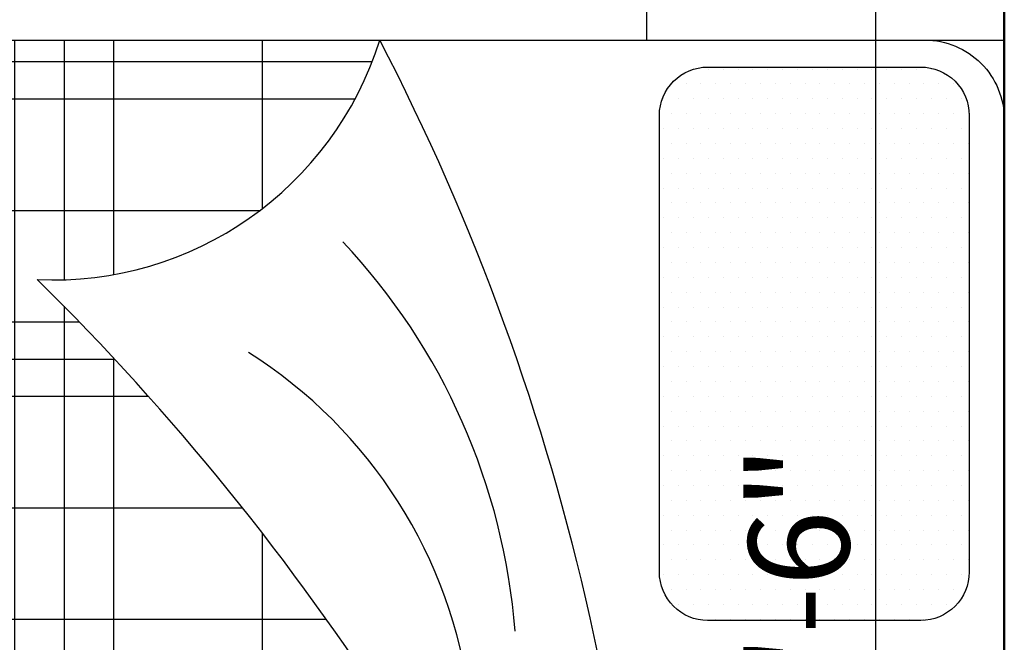
# Model space of a CAD drawing. Units: inches. Extents: x 3064 to 19385, y 846 to 15425.
# Tile 97 of 108: x 7612 to 7661, y 1063 to 1094. Entities that reach past the tile are written whole.
import ezdxf

# ---------------------------------------------------------------- set-up
doc = ezdxf.new("R2010")
doc.units = ezdxf.units.IN
for name, color, linetype, lineweight in [('A-ANNO-DIMS', 2, 'Continuous', 18), ('A-FLOR-FIXT', 9, 'Continuous', 18), ('A-WALL', 7, 'Continuous', 50)]:
    doc.layers.add(name, color=color, linetype=linetype, lineweight=lineweight)
doc.layers.add('BLOCK', color=6, linetype='Continuous')
doc.styles.get("Standard").update_dxf_attribs({"font": 'arial.ttf'})
doc.dimstyles.new('ISO-25', dxfattribs={"dimtxt": 9, "dimasz": 2.5, "dimexe": 1.25, "dimexo": 0.625, "dimtad": 1, "dimdec": 1, "dimlunit": 3, "dimtxsty": 'Standard', "dimcen": 2.5, "dimadec": 0, "dimazin": 0, "dimtfac": 1, "dimtdec": 1, "dimtmove": 0, "dimatfit": 3, "dimfxl": 1, "dimarcsym": 0})

# ---------------------------------------------------------------- blocks, each defined once
blk = doc.blocks.new('*D234')
at = {"layer": 'A-ANNO-DIMS', "color": 0, "lineweight": -2, "transparency": 16777216}
for p, q in [((7660.621, 1144.34), (7653.626, 1144.34)), ((7654.876, 984.84), (7654.876, 1141.84)), ((7660.621, 982.34), (7653.626, 982.34))]:
    blk.add_line(p, q, dxfattribs=at)
at = {"layer": 'A-ANNO-DIMS', "color": 0, "transparency": 16777216}
for points in [[(7654.459, 1141.84), (7655.292, 1141.84), (7654.876, 1144.34)], [(7654.459, 984.84), (7655.292, 984.84), (7654.876, 982.34)]]:
    blk.add_solid(points, dxfattribs=at)
at = {"layer": 'Defpoints', "color": 0, "transparency": 16777216}
for p in [(7654.876, 1144.34), (7661.246, 1144.34), (7661.246, 982.34)]:
    blk.add_point(p, dxfattribs=at)
at = {"layer": 'A-ANNO-DIMS', "color": 0, "transparency": 16777216, "insert": (7651.696, 1063.34), "char_height": 5, "attachment_point": 5, "rotation": 90}
blk.add_mtext('13\'-6"', dxfattribs=at)
blk = doc.blocks.new('*X5')
at = {"color": 0}
for p, q in [((276.598, 451.25), (280.51, 451.25)), ((275.455, 450.625), (280.51, 450.625)), ((274.411, 450), (280.51, 450)), ((265.51, 448.125), (267.634, 448.125)), ((271.723, 448.125), (280.51, 448.125)), ((265.51, 446.25), (268.465, 446.25)), ((269.519, 446.25), (280.51, 446.25)), ((265.51, 445.625), (268.531, 445.625)), ((268.866, 445.625), (280.51, 445.625)), ((265.51, 445), (280.51, 445)), ((265.51, 443.125), (280.51, 443.125)), ((265.51, 441.25), (280.51, 441.25)), ((265.51, 440.625), (280.51, 440.625)), ((265.634, 440), (280.386, 440))]:
    blk.add_line(p, q, dxfattribs=at)
blk = doc.blocks.new('*X6')
at = {"color": 0}
for p, q in [((265.781, 439.797), (265.781, 449.511)), ((266.25, 439.517), (266.25, 449.296)), ((272.812, 439.482), (272.812, 448.934)), ((267.656, 439.482), (267.656, 448.095)), ((271.406, 439.482), (271.406, 447.876)), ((270, 439.482), (270, 446.689)), ((269.531, 439.482), (269.531, 446.262)), ((269.062, 439.482), (269.062, 445.817))]:
    blk.add_line(p, q, dxfattribs=at)
blk = doc.blocks.new('*X7')
at = {"color": 0}
for p, q in [((266.4375, 457.03125), (266.4375, 457.03125)), ((266.8125, 457.03125), (266.8125, 457.03125)), ((267.1875, 457.03125), (267.1875, 457.03125)), ((267.5625, 457.03125), (267.5625, 457.03125)), ((267.9375, 457.03125), (267.9375, 457.03125)), ((268.3125, 457.03125), (268.3125, 457.03125)), ((268.6875, 457.03125), (268.6875, 457.03125)), ((269.0625, 457.03125), (269.0625, 457.03125)), ((269.4375, 457.03125), (269.4375, 457.03125)), ((269.8125, 457.03125), (269.8125, 457.03125)), ((270.1875, 457.03125), (270.1875, 457.03125)), ((270.5625, 457.03125), (270.5625, 457.03125)), ((270.9375, 457.03125), (270.9375, 457.03125)), ((271.3125, 457.03125), (271.3125, 457.03125)), ((271.6875, 457.03125), (271.6875, 457.03125)), ((272.0625, 457.03125), (272.0625, 457.03125)), ((266.25, 456.9375), (266.25, 456.9375)), ((266.625, 456.9375), (266.625, 456.9375)), ((267, 456.9375), (267, 456.9375)), ((267.375, 456.9375), (267.375, 456.9375)), ((267.75, 456.9375), (267.75, 456.9375)), ((268.125, 456.9375), (268.125, 456.9375)), ((268.5, 456.9375), (268.5, 456.9375)), ((268.875, 456.9375), (268.875, 456.9375)), ((269.25, 456.9375), (269.25, 456.9375)), ((269.625, 456.9375), (269.625, 456.9375)), ((270, 456.9375), (270, 456.9375)), ((270.375, 456.9375), (270.375, 456.9375)), ((270.75, 456.9375), (270.75, 456.9375)), ((271.125, 456.9375), (271.125, 456.9375)), ((271.5, 456.9375), (271.5, 456.9375)), ((271.875, 456.9375), (271.875, 456.9375)), ((272.25, 456.9375), (272.25, 456.9375)), ((266.0625, 456.84375), (266.0625, 456.84375)), ((266.4375, 456.84375), (266.4375, 456.84375)), ((266.8125, 456.84375), (266.8125, 456.84375)), ((267.1875, 456.84375), (267.1875, 456.84375)), ((267.5625, 456.84375), (267.5625, 456.84375)), ((267.9375, 456.84375), (267.9375, 456.84375)), ((268.3125, 456.84375), (268.3125, 456.84375)), ((268.6875, 456.84375), (268.6875, 456.84375)), ((269.0625, 456.84375), (269.0625, 456.84375)), ((269.4375, 456.84375), (269.4375, 456.84375)), ((269.8125, 456.84375), (269.8125, 456.84375)), ((270.1875, 456.84375), (270.1875, 456.84375)), ((270.5625, 456.84375), (270.5625, 456.84375)), ((270.9375, 456.84375), (270.9375, 456.84375)), ((271.3125, 456.84375), (271.3125, 456.84375)), ((271.6875, 456.84375), (271.6875, 456.84375)), ((272.0625, 456.84375), (272.0625, 456.84375)), ((272.4375, 456.84375), (272.4375, 456.84375)), ((266.0625, 456.65625), (266.0625, 456.65625)), ((266.25, 456.75), (266.25, 456.75)), ((266.4375, 456.65625), (266.4375, 456.65625)), ((266.625, 456.75), (266.625, 456.75)), ((266.8125, 456.65625), (266.8125, 456.65625)), ((267, 456.75), (267, 456.75)), ((267.1875, 456.65625), (267.1875, 456.65625)), ((267.375, 456.75), (267.375, 456.75)), ((267.5625, 456.65625), (267.5625, 456.65625)), ((267.75, 456.75), (267.75, 456.75)), ((267.9375, 456.65625), (267.9375, 456.65625)), ((268.125, 456.75), (268.125, 456.75)), ((268.3125, 456.65625), (268.3125, 456.65625)), ((268.5, 456.75), (268.5, 456.75)), ((268.6875, 456.65625), (268.6875, 456.65625)), ((268.875, 456.75), (268.875, 456.75)), ((269.0625, 456.65625), (269.0625, 456.65625)), ((269.25, 456.75), (269.25, 456.75)), ((269.4375, 456.65625), (269.4375, 456.65625)), ((269.625, 456.75), (269.625, 456.75)), ((269.8125, 456.65625), (269.8125, 456.65625)), ((270, 456.75), (270, 456.75)), ((270.1875, 456.65625), (270.1875, 456.65625)), ((270.375, 456.75), (270.375, 456.75)), ((270.5625, 456.65625), (270.5625, 456.65625)), ((270.75, 456.75), (270.75, 456.75)), ((270.9375, 456.65625), (270.9375, 456.65625)), ((271.125, 456.75), (271.125, 456.75)), ((271.3125, 456.65625), (271.3125, 456.65625)), ((271.5, 456.75), (271.5, 456.75)), ((271.6875, 456.65625), (271.6875, 456.65625)), ((271.875, 456.75), (271.875, 456.75)), ((272.0625, 456.65625), (272.0625, 456.65625)), ((272.25, 456.75), (272.25, 456.75)), ((272.4375, 456.65625), (272.4375, 456.65625)), ((272.625, 456.75), (272.625, 456.75)), ((265.875, 456.5625), (265.875, 456.5625)), ((266.25, 456.5625), (266.25, 456.5625)), ((266.625, 456.5625), (266.625, 456.5625)), ((267, 456.5625), (267, 456.5625)), ((267.375, 456.5625), (267.375, 456.5625)), ((267.75, 456.5625), (267.75, 456.5625)), ((268.125, 456.5625), (268.125, 456.5625)), ((268.5, 456.5625), (268.5, 456.5625)), ((268.875, 456.5625), (268.875, 456.5625)), ((269.25, 456.5625), (269.25, 456.5625)), ((269.625, 456.5625), (269.625, 456.5625)), ((270, 456.5625), (270, 456.5625)), ((270.375, 456.5625), (270.375, 456.5625)), ((270.75, 456.5625), (270.75, 456.5625)), ((271.125, 456.5625), (271.125, 456.5625)), ((271.5, 456.5625), (271.5, 456.5625)), ((271.875, 456.5625), (271.875, 456.5625)), ((272.25, 456.5625), (272.25, 456.5625)), ((272.625, 456.5625), (272.625, 456.5625)), ((266.0625, 456.46875), (266.0625, 456.46875)), ((266.4375, 456.46875), (266.4375, 456.46875)), ((266.8125, 456.46875), (266.8125, 456.46875)), ((267.1875, 456.46875), (267.1875, 456.46875)), ((267.5625, 456.46875), (267.5625, 456.46875)), ((267.9375, 456.46875), (267.9375, 456.46875)), ((268.3125, 456.46875), (268.3125, 456.46875)), ((268.6875, 456.46875), (268.6875, 456.46875)), ((269.0625, 456.46875), (269.0625, 456.46875)), ((269.4375, 456.46875), (269.4375, 456.46875)), ((269.8125, 456.46875), (269.8125, 456.46875)), ((270.1875, 456.46875), (270.1875, 456.46875)), ((270.5625, 456.46875), (270.5625, 456.46875)), ((270.9375, 456.46875), (270.9375, 456.46875)), ((271.3125, 456.46875), (271.3125, 456.46875)), ((271.6875, 456.46875), (271.6875, 456.46875)), ((272.0625, 456.46875), (272.0625, 456.46875)), ((272.4375, 456.46875), (272.4375, 456.46875)), ((272.8125, 456.46875), (272.8125, 456.46875)), ((265.875, 456.375), (265.875, 456.375)), ((266.25, 456.375), (266.25, 456.375)), ((266.625, 456.375), (266.625, 456.375)), ((267, 456.375), (267, 456.375)), ((267.375, 456.375), (267.375, 456.375)), ((267.75, 456.375), (267.75, 456.375)), ((268.125, 456.375), (268.125, 456.375)), ((268.5, 456.375), (268.5, 456.375)), ((268.875, 456.375), (268.875, 456.375)), ((269.25, 456.375), (269.25, 456.375)), ((269.625, 456.375), (269.625, 456.375)), ((270, 456.375), (270, 456.375)), ((270.375, 456.375), (270.375, 456.375)), ((270.75, 456.375), (270.75, 456.375)), ((271.125, 456.375), (271.125, 456.375)), ((271.5, 456.375), (271.5, 456.375)), ((271.875, 456.375), (271.875, 456.375)), ((272.25, 456.375), (272.25, 456.375)), ((272.625, 456.375), (272.625, 456.375)), ((265.875, 456.1875), (265.875, 456.1875)), ((266.0625, 456.28125), (266.0625, 456.28125)), ((266.25, 456.1875), (266.25, 456.1875)), ((266.4375, 456.28125), (266.4375, 456.28125)), ((266.625, 456.1875), (266.625, 456.1875)), ((266.8125, 456.28125), (266.8125, 456.28125)), ((267, 456.1875), (267, 456.1875)), ((267.1875, 456.28125), (267.1875, 456.28125)), ((267.375, 456.1875), (267.375, 456.1875)), ((267.5625, 456.28125), (267.5625, 456.28125)), ((267.75, 456.1875), (267.75, 456.1875)), ((267.9375, 456.28125), (267.9375, 456.28125)), ((268.125, 456.1875), (268.125, 456.1875)), ((268.3125, 456.28125), (268.3125, 456.28125)), ((268.5, 456.1875), (268.5, 456.1875)), ((268.6875, 456.28125), (268.6875, 456.28125)), ((268.875, 456.1875), (268.875, 456.1875)), ((269.0625, 456.28125), (269.0625, 456.28125)), ((269.25, 456.1875), (269.25, 456.1875)), ((269.4375, 456.28125), (269.4375, 456.28125)), ((269.625, 456.1875), (269.625, 456.1875)), ((269.8125, 456.28125), (269.8125, 456.28125)), ((270, 456.1875), (270, 456.1875)), ((270.1875, 456.28125), (270.1875, 456.28125)), ((270.375, 456.1875), (270.375, 456.1875)), ((270.5625, 456.28125), (270.5625, 456.28125)), ((270.75, 456.1875), (270.75, 456.1875)), ((270.9375, 456.28125), (270.9375, 456.28125)), ((271.125, 456.1875), (271.125, 456.1875)), ((271.3125, 456.28125), (271.3125, 456.28125)), ((271.5, 456.1875), (271.5, 456.1875)), ((271.6875, 456.28125), (271.6875, 456.28125)), ((271.875, 456.1875), (271.875, 456.1875)), ((272.0625, 456.28125), (272.0625, 456.28125)), ((272.25, 456.1875), (272.25, 456.1875)), ((272.4375, 456.28125), (272.4375, 456.28125)), ((272.625, 456.1875), (272.625, 456.1875)), ((272.8125, 456.28125), (272.8125, 456.28125)), ((266.0625, 456.09375), (266.0625, 456.09375)), ((266.4375, 456.09375), (266.4375, 456.09375)), ((266.8125, 456.09375), (266.8125, 456.09375)), ((267.1875, 456.09375), (267.1875, 456.09375)), ((267.5625, 456.09375), (267.5625, 456.09375)), ((267.9375, 456.09375), (267.9375, 456.09375)), ((268.3125, 456.09375), (268.3125, 456.09375)), ((268.6875, 456.09375), (268.6875, 456.09375)), ((269.0625, 456.09375), (269.0625, 456.09375)), ((269.4375, 456.09375), (269.4375, 456.09375)), ((269.8125, 456.09375), (269.8125, 456.09375)), ((270.1875, 456.09375), (270.1875, 456.09375)), ((270.5625, 456.09375), (270.5625, 456.09375)), ((270.9375, 456.09375), (270.9375, 456.09375)), ((271.3125, 456.09375), (271.3125, 456.09375)), ((271.6875, 456.09375), (271.6875, 456.09375)), ((272.0625, 456.09375), (272.0625, 456.09375)), ((272.4375, 456.09375), (272.4375, 456.09375)), ((272.8125, 456.09375), (272.8125, 456.09375)), ((265.875, 456), (265.875, 456)), ((266.25, 456), (266.25, 456)), ((266.625, 456), (266.625, 456)), ((267, 456), (267, 456)), ((267.375, 456), (267.375, 456)), ((267.75, 456), (267.75, 456)), ((268.125, 456), (268.125, 456)), ((268.5, 456), (268.5, 456)), ((268.875, 456), (268.875, 456)), ((269.25, 456), (269.25, 456)), ((269.625, 456), (269.625, 456)), ((270, 456), (270, 456)), ((270.375, 456), (270.375, 456)), ((270.75, 456), (270.75, 456)), ((271.125, 456), (271.125, 456)), ((271.5, 456), (271.5, 456)), ((271.875, 456), (271.875, 456)), ((272.25, 456), (272.25, 456)), ((272.625, 456), (272.625, 456)), ((265.875, 455.8125), (265.875, 455.8125)), ((266.0625, 455.90625), (266.0625, 455.90625)), ((266.25, 455.8125), (266.25, 455.8125)), ((266.4375, 455.90625), (266.4375, 455.90625)), ((266.625, 455.8125), (266.625, 455.8125)), ((266.8125, 455.90625), (266.8125, 455.90625)), ((267, 455.8125), (267, 455.8125)), ((267.1875, 455.90625), (267.1875, 455.90625)), ((267.375, 455.8125), (267.375, 455.8125)), ((267.5625, 455.90625), (267.5625, 455.90625)), ((267.75, 455.8125), (267.75, 455.8125)), ((267.9375, 455.90625), (267.9375, 455.90625)), ((268.125, 455.8125), (268.125, 455.8125)), ((268.3125, 455.90625), (268.3125, 455.90625)), ((268.5, 455.8125), (268.5, 455.8125)), ((268.6875, 455.90625), (268.6875, 455.90625)), ((268.875, 455.8125), (268.875, 455.8125)), ((269.0625, 455.90625), (269.0625, 455.90625)), ((269.25, 455.8125), (269.25, 455.8125)), ((269.4375, 455.90625), (269.4375, 455.90625)), ((269.625, 455.8125), (269.625, 455.8125)), ((269.8125, 455.90625), (269.8125, 455.90625)), ((270, 455.8125), (270, 455.8125)), ((270.1875, 455.90625), (270.1875, 455.90625)), ((270.375, 455.8125), (270.375, 455.8125)), ((270.5625, 455.90625), (270.5625, 455.90625)), ((270.75, 455.8125), (270.75, 455.8125)), ((270.9375, 455.90625), (270.9375, 455.90625)), ((271.125, 455.8125), (271.125, 455.8125)), ((271.3125, 455.90625), (271.3125, 455.90625)), ((271.5, 455.8125), (271.5, 455.8125)), ((271.6875, 455.90625), (271.6875, 455.90625)), ((271.875, 455.8125), (271.875, 455.8125)), ((272.0625, 455.90625), (272.0625, 455.90625)), ((272.25, 455.8125), (272.25, 455.8125)), ((272.4375, 455.90625), (272.4375, 455.90625)), ((272.625, 455.8125), (272.625, 455.8125)), ((272.8125, 455.90625), (272.8125, 455.90625)), ((266.0625, 455.71875), (266.0625, 455.71875)), ((266.4375, 455.71875), (266.4375, 455.71875)), ((266.8125, 455.71875), (266.8125, 455.71875)), ((267.1875, 455.71875), (267.1875, 455.71875)), ((267.5625, 455.71875), (267.5625, 455.71875)), ((267.9375, 455.71875), (267.9375, 455.71875)), ((268.3125, 455.71875), (268.3125, 455.71875)), ((268.6875, 455.71875), (268.6875, 455.71875)), ((269.0625, 455.71875), (269.0625, 455.71875)), ((269.4375, 455.71875), (269.4375, 455.71875)), ((269.8125, 455.71875), (269.8125, 455.71875)), ((270.1875, 455.71875), (270.1875, 455.71875)), ((270.5625, 455.71875), (270.5625, 455.71875)), ((270.9375, 455.71875), (270.9375, 455.71875)), ((271.3125, 455.71875), (271.3125, 455.71875)), ((271.6875, 455.71875), (271.6875, 455.71875)), ((272.0625, 455.71875), (272.0625, 455.71875)), ((272.4375, 455.71875), (272.4375, 455.71875)), ((272.8125, 455.71875), (272.8125, 455.71875)), ((265.875, 455.625), (265.875, 455.625)), ((266.25, 455.625), (266.25, 455.625)), ((266.625, 455.625), (266.625, 455.625)), ((267, 455.625), (267, 455.625)), ((267.375, 455.625), (267.375, 455.625)), ((267.75, 455.625), (267.75, 455.625)), ((268.125, 455.625), (268.125, 455.625)), ((268.5, 455.625), (268.5, 455.625)), ((268.875, 455.625), (268.875, 455.625)), ((269.25, 455.625), (269.25, 455.625)), ((269.625, 455.625), (269.625, 455.625)), ((270, 455.625), (270, 455.625)), ((270.375, 455.625), (270.375, 455.625)), ((270.75, 455.625), (270.75, 455.625)), ((271.125, 455.625), (271.125, 455.625)), ((271.5, 455.625), (271.5, 455.625)), ((271.875, 455.625), (271.875, 455.625)), ((272.25, 455.625), (272.25, 455.625)), ((272.625, 455.625), (272.625, 455.625)), ((265.875, 455.4375), (265.875, 455.4375)), ((266.0625, 455.53125), (266.0625, 455.53125)), ((266.25, 455.4375), (266.25, 455.4375)), ((266.4375, 455.53125), (266.4375, 455.53125)), ((266.625, 455.4375), (266.625, 455.4375)), ((266.8125, 455.53125), (266.8125, 455.53125)), ((267, 455.4375), (267, 455.4375)), ((267.1875, 455.53125), (267.1875, 455.53125)), ((267.375, 455.4375), (267.375, 455.4375)), ((267.5625, 455.53125), (267.5625, 455.53125)), ((267.75, 455.4375), (267.75, 455.4375)), ((267.9375, 455.53125), (267.9375, 455.53125)), ((268.125, 455.4375), (268.125, 455.4375)), ((268.3125, 455.53125), (268.3125, 455.53125)), ((268.5, 455.4375), (268.5, 455.4375)), ((268.6875, 455.53125), (268.6875, 455.53125)), ((268.875, 455.4375), (268.875, 455.4375)), ((269.0625, 455.53125), (269.0625, 455.53125)), ((269.25, 455.4375), (269.25, 455.4375)), ((269.4375, 455.53125), (269.4375, 455.53125)), ((269.625, 455.4375), (269.625, 455.4375)), ((269.8125, 455.53125), (269.8125, 455.53125)), ((270, 455.4375), (270, 455.4375)), ((270.1875, 455.53125), (270.1875, 455.53125)), ((270.375, 455.4375), (270.375, 455.4375)), ((270.5625, 455.53125), (270.5625, 455.53125)), ((270.75, 455.4375), (270.75, 455.4375)), ((270.9375, 455.53125), (270.9375, 455.53125)), ((271.125, 455.4375), (271.125, 455.4375)), ((271.3125, 455.53125), (271.3125, 455.53125)), ((271.5, 455.4375), (271.5, 455.4375)), ((271.6875, 455.53125), (271.6875, 455.53125)), ((271.875, 455.4375), (271.875, 455.4375)), ((272.0625, 455.53125), (272.0625, 455.53125)), ((272.25, 455.4375), (272.25, 455.4375)), ((272.4375, 455.53125), (272.4375, 455.53125)), ((272.625, 455.4375), (272.625, 455.4375)), ((272.8125, 455.53125), (272.8125, 455.53125)), ((266.0625, 455.34375), (266.0625, 455.34375)), ((266.4375, 455.34375), (266.4375, 455.34375)), ((266.8125, 455.34375), (266.8125, 455.34375)), ((267.1875, 455.34375), (267.1875, 455.34375)), ((267.5625, 455.34375), (267.5625, 455.34375)), ((267.9375, 455.34375), (267.9375, 455.34375)), ((268.3125, 455.34375), (268.3125, 455.34375)), ((268.6875, 455.34375), (268.6875, 455.34375)), ((269.0625, 455.34375), (269.0625, 455.34375)), ((269.4375, 455.34375), (269.4375, 455.34375)), ((269.8125, 455.34375), (269.8125, 455.34375)), ((270.1875, 455.34375), (270.1875, 455.34375)), ((270.5625, 455.34375), (270.5625, 455.34375)), ((270.9375, 455.34375), (270.9375, 455.34375)), ((271.3125, 455.34375), (271.3125, 455.34375)), ((271.6875, 455.34375), (271.6875, 455.34375)), ((272.0625, 455.34375), (272.0625, 455.34375)), ((272.4375, 455.34375), (272.4375, 455.34375)), ((272.8125, 455.34375), (272.8125, 455.34375)), ((265.875, 455.25), (265.875, 455.25)), ((266.25, 455.25), (266.25, 455.25)), ((266.625, 455.25), (266.625, 455.25)), ((267, 455.25), (267, 455.25)), ((267.375, 455.25), (267.375, 455.25)), ((267.75, 455.25), (267.75, 455.25)), ((268.125, 455.25), (268.125, 455.25)), ((268.5, 455.25), (268.5, 455.25)), ((268.875, 455.25), (268.875, 455.25)), ((269.25, 455.25), (269.25, 455.25)), ((269.625, 455.25), (269.625, 455.25)), ((270, 455.25), (270, 455.25)), ((270.375, 455.25), (270.375, 455.25)), ((270.75, 455.25), (270.75, 455.25)), ((271.125, 455.25), (271.125, 455.25)), ((271.5, 455.25), (271.5, 455.25)), ((271.875, 455.25), (271.875, 455.25)), ((272.25, 455.25), (272.25, 455.25)), ((272.625, 455.25), (272.625, 455.25)), ((265.875, 455.0625), (265.875, 455.0625)), ((266.0625, 455.15625), (266.0625, 455.15625)), ((266.25, 455.0625), (266.25, 455.0625)), ((266.4375, 455.15625), (266.4375, 455.15625)), ((266.625, 455.0625), (266.625, 455.0625)), ((266.8125, 455.15625), (266.8125, 455.15625)), ((267, 455.0625), (267, 455.0625)), ((267.1875, 455.15625), (267.1875, 455.15625)), ((267.375, 455.0625), (267.375, 455.0625)), ((267.5625, 455.15625), (267.5625, 455.15625)), ((267.75, 455.0625), (267.75, 455.0625)), ((267.9375, 455.15625), (267.9375, 455.15625)), ((268.125, 455.0625), (268.125, 455.0625)), ((268.3125, 455.15625), (268.3125, 455.15625)), ((268.5, 455.0625), (268.5, 455.0625)), ((268.6875, 455.15625), (268.6875, 455.15625)), ((268.875, 455.0625), (268.875, 455.0625)), ((269.0625, 455.15625), (269.0625, 455.15625)), ((269.25, 455.0625), (269.25, 455.0625)), ((269.4375, 455.15625), (269.4375, 455.15625)), ((269.625, 455.0625), (269.625, 455.0625)), ((269.8125, 455.15625), (269.8125, 455.15625)), ((270, 455.0625), (270, 455.0625)), ((270.1875, 455.15625), (270.1875, 455.15625)), ((270.375, 455.0625), (270.375, 455.0625)), ((270.5625, 455.15625), (270.5625, 455.15625)), ((270.75, 455.0625), (270.75, 455.0625)), ((270.9375, 455.15625), (270.9375, 455.15625)), ((271.125, 455.0625), (271.125, 455.0625)), ((271.3125, 455.15625), (271.3125, 455.15625)), ((271.5, 455.0625), (271.5, 455.0625)), ((271.6875, 455.15625), (271.6875, 455.15625)), ((271.875, 455.0625), (271.875, 455.0625)), ((272.0625, 455.15625), (272.0625, 455.15625)), ((272.25, 455.0625), (272.25, 455.0625)), ((272.4375, 455.15625), (272.4375, 455.15625)), ((272.625, 455.0625), (272.625, 455.0625)), ((272.8125, 455.15625), (272.8125, 455.15625)), ((266.0625, 454.96875), (266.0625, 454.96875)), ((266.4375, 454.96875), (266.4375, 454.96875)), ((266.8125, 454.96875), (266.8125, 454.96875)), ((267.1875, 454.96875), (267.1875, 454.96875)), ((267.5625, 454.96875), (267.5625, 454.96875)), ((267.9375, 454.96875), (267.9375, 454.96875)), ((268.3125, 454.96875), (268.3125, 454.96875)), ((268.6875, 454.96875), (268.6875, 454.96875)), ((269.0625, 454.96875), (269.0625, 454.96875)), ((269.4375, 454.96875), (269.4375, 454.96875)), ((269.8125, 454.96875), (269.8125, 454.96875)), ((270.1875, 454.96875), (270.1875, 454.96875)), ((270.5625, 454.96875), (270.5625, 454.96875)), ((270.9375, 454.96875), (270.9375, 454.96875)), ((271.3125, 454.96875), (271.3125, 454.96875)), ((271.6875, 454.96875), (271.6875, 454.96875)), ((272.0625, 454.96875), (272.0625, 454.96875)), ((272.4375, 454.96875), (272.4375, 454.96875)), ((272.8125, 454.96875), (272.8125, 454.96875)), ((265.875, 454.875), (265.875, 454.875)), ((266.25, 454.875), (266.25, 454.875)), ((266.625, 454.875), (266.625, 454.875)), ((267, 454.875), (267, 454.875)), ((267.375, 454.875), (267.375, 454.875)), ((267.75, 454.875), (267.75, 454.875)), ((268.125, 454.875), (268.125, 454.875)), ((268.5, 454.875), (268.5, 454.875)), ((268.875, 454.875), (268.875, 454.875)), ((269.25, 454.875), (269.25, 454.875)), ((269.625, 454.875), (269.625, 454.875)), ((270, 454.875), (270, 454.875)), ((270.375, 454.875), (270.375, 454.875)), ((270.75, 454.875), (270.75, 454.875)), ((271.125, 454.875), (271.125, 454.875)), ((271.5, 454.875), (271.5, 454.875)), ((271.875, 454.875), (271.875, 454.875)), ((272.25, 454.875), (272.25, 454.875)), ((272.625, 454.875), (272.625, 454.875)), ((265.875, 454.6875), (265.875, 454.6875)), ((266.0625, 454.78125), (266.0625, 454.78125)), ((266.25, 454.6875), (266.25, 454.6875)), ((266.4375, 454.78125), (266.4375, 454.78125)), ((266.625, 454.6875), (266.625, 454.6875)), ((266.8125, 454.78125), (266.8125, 454.78125)), ((267, 454.6875), (267, 454.6875)), ((267.1875, 454.78125), (267.1875, 454.78125)), ((267.375, 454.6875), (267.375, 454.6875)), ((267.5625, 454.78125), (267.5625, 454.78125)), ((267.75, 454.6875), (267.75, 454.6875)), ((267.9375, 454.78125), (267.9375, 454.78125)), ((268.125, 454.6875), (268.125, 454.6875)), ((268.3125, 454.78125), (268.3125, 454.78125)), ((268.5, 454.6875), (268.5, 454.6875)), ((268.6875, 454.78125), (268.6875, 454.78125)), ((268.875, 454.6875), (268.875, 454.6875)), ((269.0625, 454.78125), (269.0625, 454.78125)), ((269.25, 454.6875), (269.25, 454.6875)), ((269.4375, 454.78125), (269.4375, 454.78125)), ((269.625, 454.6875), (269.625, 454.6875)), ((269.8125, 454.78125), (269.8125, 454.78125)), ((270, 454.6875), (270, 454.6875)), ((270.1875, 454.78125), (270.1875, 454.78125)), ((270.375, 454.6875), (270.375, 454.6875)), ((270.5625, 454.78125), (270.5625, 454.78125)), ((270.75, 454.6875), (270.75, 454.6875)), ((270.9375, 454.78125), (270.9375, 454.78125)), ((271.125, 454.6875), (271.125, 454.6875)), ((271.3125, 454.78125), (271.3125, 454.78125)), ((271.5, 454.6875), (271.5, 454.6875)), ((271.6875, 454.78125), (271.6875, 454.78125)), ((271.875, 454.6875), (271.875, 454.6875)), ((272.0625, 454.78125), (272.0625, 454.78125)), ((272.25, 454.6875), (272.25, 454.6875)), ((272.4375, 454.78125), (272.4375, 454.78125)), ((272.625, 454.6875), (272.625, 454.6875)), ((272.8125, 454.78125), (272.8125, 454.78125)), ((266.0625, 454.59375), (266.0625, 454.59375)), ((266.4375, 454.59375), (266.4375, 454.59375)), ((266.8125, 454.59375), (266.8125, 454.59375)), ((267.1875, 454.59375), (267.1875, 454.59375)), ((267.5625, 454.59375), (267.5625, 454.59375)), ((267.9375, 454.59375), (267.9375, 454.59375)), ((268.3125, 454.59375), (268.3125, 454.59375)), ((268.6875, 454.59375), (268.6875, 454.59375)), ((269.0625, 454.59375), (269.0625, 454.59375)), ((269.4375, 454.59375), (269.4375, 454.59375)), ((269.8125, 454.59375), (269.8125, 454.59375)), ((270.1875, 454.59375), (270.1875, 454.59375)), ((270.5625, 454.59375), (270.5625, 454.59375)), ((270.9375, 454.59375), (270.9375, 454.59375)), ((271.3125, 454.59375), (271.3125, 454.59375)), ((271.6875, 454.59375), (271.6875, 454.59375)), ((272.0625, 454.59375), (272.0625, 454.59375)), ((272.4375, 454.59375), (272.4375, 454.59375)), ((272.8125, 454.59375), (272.8125, 454.59375)), ((265.875, 454.5), (265.875, 454.5)), ((266.25, 454.5), (266.25, 454.5)), ((266.625, 454.5), (266.625, 454.5)), ((267, 454.5), (267, 454.5)), ((267.375, 454.5), (267.375, 454.5)), ((267.75, 454.5), (267.75, 454.5)), ((268.125, 454.5), (268.125, 454.5)), ((268.5, 454.5), (268.5, 454.5)), ((268.875, 454.5), (268.875, 454.5)), ((269.25, 454.5), (269.25, 454.5)), ((269.625, 454.5), (269.625, 454.5)), ((270, 454.5), (270, 454.5)), ((270.375, 454.5), (270.375, 454.5)), ((270.75, 454.5), (270.75, 454.5)), ((271.125, 454.5), (271.125, 454.5)), ((271.5, 454.5), (271.5, 454.5)), ((271.875, 454.5), (271.875, 454.5)), ((272.25, 454.5), (272.25, 454.5)), ((272.625, 454.5), (272.625, 454.5)), ((265.875, 454.3125), (265.875, 454.3125)), ((266.0625, 454.40625), (266.0625, 454.40625)), ((266.25, 454.3125), (266.25, 454.3125)), ((266.4375, 454.40625), (266.4375, 454.40625)), ((266.625, 454.3125), (266.625, 454.3125)), ((266.8125, 454.40625), (266.8125, 454.40625)), ((267, 454.3125), (267, 454.3125)), ((267.1875, 454.40625), (267.1875, 454.40625)), ((267.375, 454.3125), (267.375, 454.3125)), ((267.5625, 454.40625), (267.5625, 454.40625)), ((267.75, 454.3125), (267.75, 454.3125)), ((267.9375, 454.40625), (267.9375, 454.40625)), ((268.125, 454.3125), (268.125, 454.3125)), ((268.3125, 454.40625), (268.3125, 454.40625)), ((268.5, 454.3125), (268.5, 454.3125)), ((268.6875, 454.40625), (268.6875, 454.40625)), ((268.875, 454.3125), (268.875, 454.3125)), ((269.0625, 454.40625), (269.0625, 454.40625)), ((269.25, 454.3125), (269.25, 454.3125)), ((269.4375, 454.40625), (269.4375, 454.40625)), ((269.625, 454.3125), (269.625, 454.3125)), ((269.8125, 454.40625), (269.8125, 454.40625)), ((270, 454.3125), (270, 454.3125)), ((270.1875, 454.40625), (270.1875, 454.40625)), ((270.375, 454.3125), (270.375, 454.3125)), ((270.5625, 454.40625), (270.5625, 454.40625)), ((270.75, 454.3125), (270.75, 454.3125)), ((270.9375, 454.40625), (270.9375, 454.40625)), ((271.125, 454.3125), (271.125, 454.3125)), ((271.3125, 454.40625), (271.3125, 454.40625)), ((271.5, 454.3125), (271.5, 454.3125)), ((271.6875, 454.40625), (271.6875, 454.40625)), ((271.875, 454.3125), (271.875, 454.3125)), ((272.0625, 454.40625), (272.0625, 454.40625)), ((272.25, 454.3125), (272.25, 454.3125)), ((272.4375, 454.40625), (272.4375, 454.40625)), ((272.625, 454.3125), (272.625, 454.3125)), ((272.8125, 454.40625), (272.8125, 454.40625)), ((266.0625, 454.21875), (266.0625, 454.21875)), ((266.4375, 454.21875), (266.4375, 454.21875)), ((266.8125, 454.21875), (266.8125, 454.21875)), ((267.1875, 454.21875), (267.1875, 454.21875)), ((267.5625, 454.21875), (267.5625, 454.21875)), ((267.9375, 454.21875), (267.9375, 454.21875)), ((268.3125, 454.21875), (268.3125, 454.21875)), ((268.6875, 454.21875), (268.6875, 454.21875)), ((269.0625, 454.21875), (269.0625, 454.21875)), ((269.4375, 454.21875), (269.4375, 454.21875)), ((269.8125, 454.21875), (269.8125, 454.21875)), ((270.1875, 454.21875), (270.1875, 454.21875)), ((270.5625, 454.21875), (270.5625, 454.21875)), ((270.9375, 454.21875), (270.9375, 454.21875)), ((271.3125, 454.21875), (271.3125, 454.21875)), ((271.6875, 454.21875), (271.6875, 454.21875)), ((272.0625, 454.21875), (272.0625, 454.21875)), ((272.4375, 454.21875), (272.4375, 454.21875)), ((272.8125, 454.21875), (272.8125, 454.21875)), ((265.875, 454.125), (265.875, 454.125)), ((266.25, 454.125), (266.25, 454.125)), ((266.625, 454.125), (266.625, 454.125)), ((267, 454.125), (267, 454.125)), ((267.375, 454.125), (267.375, 454.125)), ((267.75, 454.125), (267.75, 454.125)), ((268.125, 454.125), (268.125, 454.125)), ((268.5, 454.125), (268.5, 454.125)), ((268.875, 454.125), (268.875, 454.125)), ((269.25, 454.125), (269.25, 454.125)), ((269.625, 454.125), (269.625, 454.125)), ((270, 454.125), (270, 454.125)), ((270.375, 454.125), (270.375, 454.125)), ((270.75, 454.125), (270.75, 454.125)), ((271.125, 454.125), (271.125, 454.125)), ((271.5, 454.125), (271.5, 454.125)), ((271.875, 454.125), (271.875, 454.125)), ((272.25, 454.125), (272.25, 454.125)), ((272.625, 454.125), (272.625, 454.125)), ((265.875, 453.9375), (265.875, 453.9375)), ((266.0625, 454.03125), (266.0625, 454.03125)), ((266.25, 453.9375), (266.25, 453.9375)), ((266.4375, 454.03125), (266.4375, 454.03125)), ((266.625, 453.9375), (266.625, 453.9375)), ((266.8125, 454.03125), (266.8125, 454.03125)), ((267, 453.9375), (267, 453.9375)), ((267.1875, 454.03125), (267.1875, 454.03125)), ((267.375, 453.9375), (267.375, 453.9375)), ((267.5625, 454.03125), (267.5625, 454.03125)), ((267.75, 453.9375), (267.75, 453.9375)), ((267.9375, 454.03125), (267.9375, 454.03125)), ((268.125, 453.9375), (268.125, 453.9375)), ((268.3125, 454.03125), (268.3125, 454.03125)), ((268.5, 453.9375), (268.5, 453.9375)), ((268.6875, 454.03125), (268.6875, 454.03125)), ((268.875, 453.9375), (268.875, 453.9375)), ((269.0625, 454.03125), (269.0625, 454.03125)), ((269.25, 453.9375), (269.25, 453.9375)), ((269.4375, 454.03125), (269.4375, 454.03125)), ((269.625, 453.9375), (269.625, 453.9375)), ((269.8125, 454.03125), (269.8125, 454.03125)), ((270, 453.9375), (270, 453.9375)), ((270.1875, 454.03125), (270.1875, 454.03125)), ((270.375, 453.9375), (270.375, 453.9375)), ((270.5625, 454.03125), (270.5625, 454.03125)), ((270.75, 453.9375), (270.75, 453.9375)), ((270.9375, 454.03125), (270.9375, 454.03125)), ((271.125, 453.9375), (271.125, 453.9375)), ((271.3125, 454.03125), (271.3125, 454.03125)), ((271.5, 453.9375), (271.5, 453.9375)), ((271.6875, 454.03125), (271.6875, 454.03125)), ((271.875, 453.9375), (271.875, 453.9375)), ((272.0625, 454.03125), (272.0625, 454.03125)), ((272.25, 453.9375), (272.25, 453.9375)), ((272.4375, 454.03125), (272.4375, 454.03125)), ((272.625, 453.9375), (272.625, 453.9375)), ((272.8125, 454.03125), (272.8125, 454.03125)), ((266.0625, 453.84375), (266.0625, 453.84375)), ((266.4375, 453.84375), (266.4375, 453.84375)), ((266.8125, 453.84375), (266.8125, 453.84375)), ((267.1875, 453.84375), (267.1875, 453.84375)), ((267.5625, 453.84375), (267.5625, 453.84375)), ((267.9375, 453.84375), (267.9375, 453.84375)), ((268.3125, 453.84375), (268.3125, 453.84375)), ((268.6875, 453.84375), (268.6875, 453.84375)), ((269.0625, 453.84375), (269.0625, 453.84375)), ((269.4375, 453.84375), (269.4375, 453.84375)), ((269.8125, 453.84375), (269.8125, 453.84375)), ((270.1875, 453.84375), (270.1875, 453.84375)), ((270.5625, 453.84375), (270.5625, 453.84375)), ((270.9375, 453.84375), (270.9375, 453.84375)), ((271.3125, 453.84375), (271.3125, 453.84375)), ((271.6875, 453.84375), (271.6875, 453.84375)), ((272.0625, 453.84375), (272.0625, 453.84375)), ((272.4375, 453.84375), (272.4375, 453.84375)), ((272.8125, 453.84375), (272.8125, 453.84375)), ((265.875, 453.75), (265.875, 453.75)), ((266.25, 453.75), (266.25, 453.75)), ((266.625, 453.75), (266.625, 453.75)), ((267, 453.75), (267, 453.75)), ((267.375, 453.75), (267.375, 453.75)), ((267.75, 453.75), (267.75, 453.75)), ((268.125, 453.75), (268.125, 453.75)), ((268.5, 453.75), (268.5, 453.75)), ((268.875, 453.75), (268.875, 453.75)), ((269.25, 453.75), (269.25, 453.75)), ((269.625, 453.75), (269.625, 453.75)), ((270, 453.75), (270, 453.75)), ((270.375, 453.75), (270.375, 453.75)), ((270.75, 453.75), (270.75, 453.75)), ((271.125, 453.75), (271.125, 453.75)), ((271.5, 453.75), (271.5, 453.75)), ((271.875, 453.75), (271.875, 453.75)), ((272.25, 453.75), (272.25, 453.75)), ((272.625, 453.75), (272.625, 453.75)), ((266.0625, 453.65625), (266.0625, 453.65625)), ((266.25, 453.5625), (266.25, 453.5625)), ((266.4375, 453.65625), (266.4375, 453.65625)), ((266.625, 453.5625), (266.625, 453.5625)), ((266.8125, 453.65625), (266.8125, 453.65625)), ((267, 453.5625), (267, 453.5625)), ((267.1875, 453.65625), (267.1875, 453.65625)), ((267.375, 453.5625), (267.375, 453.5625)), ((267.5625, 453.65625), (267.5625, 453.65625)), ((267.75, 453.5625), (267.75, 453.5625)), ((267.9375, 453.65625), (267.9375, 453.65625)), ((268.125, 453.5625), (268.125, 453.5625)), ((268.3125, 453.65625), (268.3125, 453.65625)), ((268.5, 453.5625), (268.5, 453.5625)), ((268.6875, 453.65625), (268.6875, 453.65625)), ((268.875, 453.5625), (268.875, 453.5625)), ((269.0625, 453.65625), (269.0625, 453.65625)), ((269.25, 453.5625), (269.25, 453.5625)), ((269.4375, 453.65625), (269.4375, 453.65625)), ((269.625, 453.5625), (269.625, 453.5625)), ((269.8125, 453.65625), (269.8125, 453.65625)), ((270, 453.5625), (270, 453.5625)), ((270.1875, 453.65625), (270.1875, 453.65625)), ((270.375, 453.5625), (270.375, 453.5625)), ((270.5625, 453.65625), (270.5625, 453.65625)), ((270.75, 453.5625), (270.75, 453.5625)), ((270.9375, 453.65625), (270.9375, 453.65625)), ((271.125, 453.5625), (271.125, 453.5625)), ((271.3125, 453.65625), (271.3125, 453.65625)), ((271.5, 453.5625), (271.5, 453.5625)), ((271.6875, 453.65625), (271.6875, 453.65625)), ((271.875, 453.5625), (271.875, 453.5625)), ((272.0625, 453.65625), (272.0625, 453.65625)), ((272.25, 453.5625), (272.25, 453.5625)), ((272.4375, 453.65625), (272.4375, 453.65625)), ((272.625, 453.5625), (272.625, 453.5625)), ((272.8125, 453.65625), (272.8125, 453.65625)), ((266.0625, 453.46875), (266.0625, 453.46875)), ((266.4375, 453.46875), (266.4375, 453.46875)), ((266.8125, 453.46875), (266.8125, 453.46875)), ((267.1875, 453.46875), (267.1875, 453.46875)), ((267.5625, 453.46875), (267.5625, 453.46875)), ((267.9375, 453.46875), (267.9375, 453.46875)), ((268.3125, 453.46875), (268.3125, 453.46875)), ((268.6875, 453.46875), (268.6875, 453.46875)), ((269.0625, 453.46875), (269.0625, 453.46875)), ((269.4375, 453.46875), (269.4375, 453.46875)), ((269.8125, 453.46875), (269.8125, 453.46875)), ((270.1875, 453.46875), (270.1875, 453.46875)), ((270.5625, 453.46875), (270.5625, 453.46875)), ((270.9375, 453.46875), (270.9375, 453.46875)), ((271.3125, 453.46875), (271.3125, 453.46875)), ((271.6875, 453.46875), (271.6875, 453.46875)), ((272.0625, 453.46875), (272.0625, 453.46875)), ((272.4375, 453.46875), (272.4375, 453.46875)), ((266.25, 453.375), (266.25, 453.375)), ((266.625, 453.375), (266.625, 453.375)), ((267, 453.375), (267, 453.375)), ((267.375, 453.375), (267.375, 453.375)), ((267.75, 453.375), (267.75, 453.375)), ((268.125, 453.375), (268.125, 453.375)), ((268.5, 453.375), (268.5, 453.375)), ((268.875, 453.375), (268.875, 453.375)), ((269.25, 453.375), (269.25, 453.375)), ((269.625, 453.375), (269.625, 453.375)), ((270, 453.375), (270, 453.375)), ((270.375, 453.375), (270.375, 453.375)), ((270.75, 453.375), (270.75, 453.375)), ((271.125, 453.375), (271.125, 453.375)), ((271.5, 453.375), (271.5, 453.375)), ((271.875, 453.375), (271.875, 453.375)), ((272.25, 453.375), (272.25, 453.375)), ((272.625, 453.375), (272.625, 453.375)), ((266.0625, 453.28125), (266.0625, 453.28125)), ((266.25, 453.1875), (266.25, 453.1875)), ((266.4375, 453.28125), (266.4375, 453.28125)), ((266.625, 453.1875), (266.625, 453.1875)), ((266.8125, 453.28125), (266.8125, 453.28125)), ((267, 453.1875), (267, 453.1875)), ((267.1875, 453.28125), (267.1875, 453.28125)), ((267.375, 453.1875), (267.375, 453.1875)), ((267.5625, 453.28125), (267.5625, 453.28125)), ((267.75, 453.1875), (267.75, 453.1875)), ((267.9375, 453.28125), (267.9375, 453.28125)), ((268.125, 453.1875), (268.125, 453.1875)), ((268.3125, 453.28125), (268.3125, 453.28125)), ((268.5, 453.1875), (268.5, 453.1875)), ((268.6875, 453.28125), (268.6875, 453.28125)), ((268.875, 453.1875), (268.875, 453.1875)), ((269.0625, 453.28125), (269.0625, 453.28125)), ((269.25, 453.1875), (269.25, 453.1875)), ((269.4375, 453.28125), (269.4375, 453.28125)), ((269.625, 453.1875), (269.625, 453.1875)), ((269.8125, 453.28125), (269.8125, 453.28125)), ((270, 453.1875), (270, 453.1875)), ((270.1875, 453.28125), (270.1875, 453.28125)), ((270.375, 453.1875), (270.375, 453.1875)), ((270.5625, 453.28125), (270.5625, 453.28125)), ((270.75, 453.1875), (270.75, 453.1875)), ((270.9375, 453.28125), (270.9375, 453.28125)), ((271.125, 453.1875), (271.125, 453.1875)), ((271.3125, 453.28125), (271.3125, 453.28125)), ((271.5, 453.1875), (271.5, 453.1875)), ((271.6875, 453.28125), (271.6875, 453.28125)), ((271.875, 453.1875), (271.875, 453.1875)), ((272.0625, 453.28125), (272.0625, 453.28125)), ((272.25, 453.1875), (272.25, 453.1875)), ((272.4375, 453.28125), (272.4375, 453.28125))]:
    blk.add_line(p, q, dxfattribs=at)
blk = doc.blocks.new('A$C52E67D0D')
at = {"layer": 'BLOCK'}
blk.add_lwpolyline([(501, 1348.6), (501, 1799.6), (0, 1799.6), (0, 1348.6)], close=True, dxfattribs=at)
for points in [[(1901, 0), (601, 0, -0.414214), (501, 100), (501, 1700, -0.414214), (601, 1800), (1901, 1800, -0.414214), (2001, 1700), (2001, 100, -0.414214)], [(1171.8, 1365.1), (595.8, 1365.1, -0.414214), (535, 1425.9), (535, 1694.8, -0.414214), (595.8, 1755.7), (1171.8, 1755.7, -0.414214), (1232.6, 1694.8), (1232.6, 1425.9, -0.414214)]]:
    blk.add_lwpolyline(points, format="xyb", close=True, dxfattribs=at)
for centre, radius, start, end in [((1888.6, -1664.5), 3015.3, 87.8642, 117.4001), ((3101, -1685.8), 3227.7, 109.926, 135.3977), ((1308.8, 377.9), 807.6, 94.4436, 133.2788), ((1410.8, 520.2), 610.8, 97.2157, 147.6656), ((371.4, 600.4), 432, 357.3792, 72.5379)]:
    blk.add_arc(centre, radius, start, end, dxfattribs=at)
at = {"layer": 'BLOCK', "xscale": 100, "yscale": 100, "zscale": 100}
for name in ['*X7', '*X6', '*X5']:
    blk.add_blockref(name, (-26050, -43948.2), dxfattribs=at)

msp = doc.modelspace()

# ---------------------------------------------------------------- linework, layer by layer
at = {"layer": 'A-WALL'}
msp.add_line((7661.246, 1144.34), (7661.246, 982.34), dxfattribs=at)

# ---------------------------------------------------------------- block references
at = {"layer": 'A-FLOR-FIXT', "xscale": 0.039370099999992, "yscale": 0.039370099999992, "zscale": 0.039370099999992, "rotation": 270}
msp.add_blockref('A$C52E67D0D', (7590.38, 1112.592), dxfattribs=at)

# ---------------------------------------------------------------- dimensions: what is measured, and where the dimension line sits
at = {"layer": 'A-ANNO-DIMS'}
dim = msp.add_linear_dim(base=(7654.876, 1144.34), p1=(7661.246, 982.34), p2=(7661.246, 1144.34), angle=90, dimstyle='ISO-25', override={"dimtxt": 5, "dimclrd": 0, "dimclre": 0, "dimclrt": 0}, dxfattribs=at)
dim.commit()
dim.dimension.update_dxf_attribs({"geometry": '*D234', "text_midpoint": (7651.696, 1063.34)})

doc.saveas('drawing.dxf')
